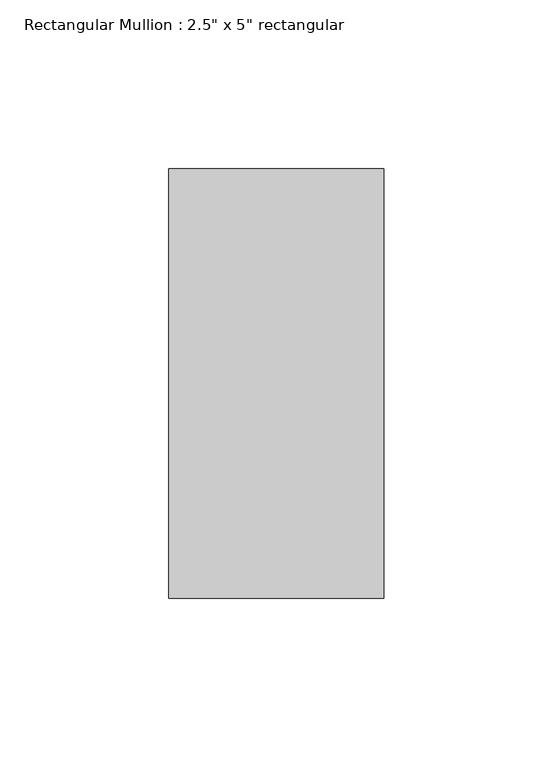
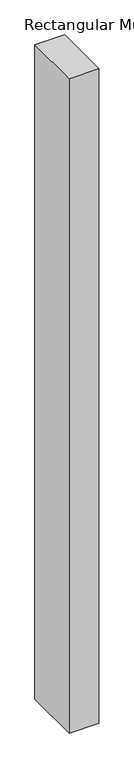
"""IFC4 building model written with IfcOpenShell, lengths in millimetres: member geometry."""

from ifc_helpers import new_model, si_unit, frame, origin, place, context, project, spatial, polyline, outline, extrude, source, transform, mapped, element, save


def member_70b51cdd(model_context):
    return source(origin(), model_context, "Body", "SweptSolid", [
        extrude(outline(polyline([(0.0, 63.5), (0.0, -63.5), (-63.5, -63.5), (-63.5, 63.5), (0.0, 63.5)])), frame((0.0, 0.0, -1478.7314865), z_axis=(0.0, 0.0, 1.0), x_axis=(1.0, 0.0, 0.0)), (0.0, 0.0, 1.0), 1478.7314865),
    ])


if __name__ == "__main__":
    model = new_model("IFC4")
    model_context = context("Model", 3, world=origin())
    ifc_project = project(units=[si_unit("LENGTHUNIT", "METRE", prefix="MILLI")], contexts=[model_context])
    site = spatial("IfcSite", under=ifc_project)
    building = spatial("IfcBuilding", under=site)
    placement = place(None, origin())
    member_shape = member_70b51cdd(model_context)
    element("IfcMember", 1, ObjectType="Rectangular Mullion : 2.5\" x 5\" rectangular", at=placement, inside=building, context=model_context, shape_type="MappedRepresentation", body=[
        mapped(member_shape, transform((0.0, 0.0, 0.0), x_axis=(1.0, 0.0, 0.0), y_axis=(0.0, 1.0, 0.0), z_axis=(0.0, 0.0, 1.0))),
    ])
    save(model, "model.ifc")

# Revit data of these elements
# Type "Rectangular Mullion : 2.5\" x 5\" rectangular"
#   built-in parameter 1007304 = 0.416667 (stored number, unit not read)
#   built-in parameter 1007301 = 0.104167 (stored number, unit not read)
#   built-in parameter 1007300 = 0.104167 (stored number, unit not read)
# Element 1 (IfcMember, "Rectangular Mullion : 2.5\" x 5\" rectangular")
#   Materials on its faces: "Aluminum"
# Materials
#   "Aluminum": class "Metal", colour RGB 247 247 247, transparency 0, Description = "Aluminum 6061", Cost = 0
